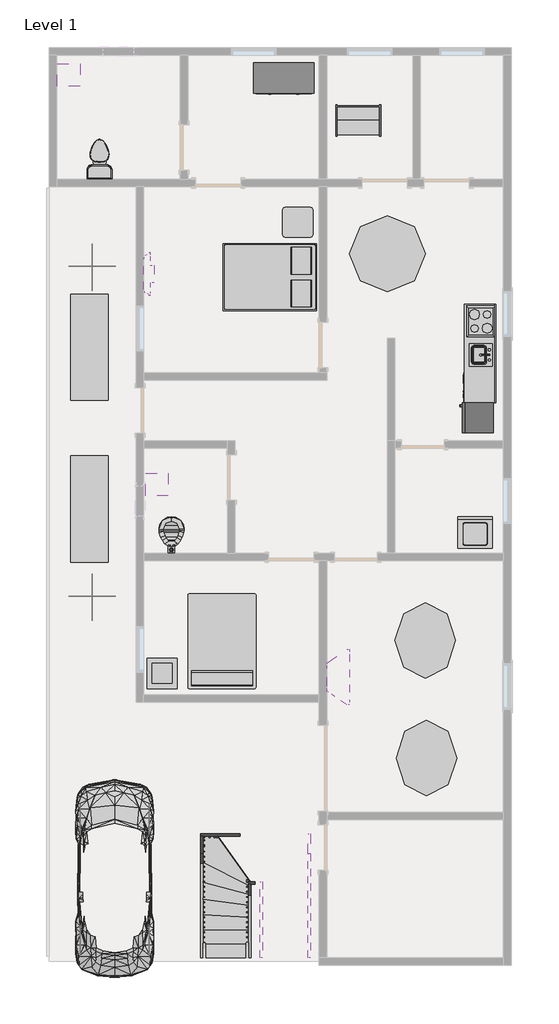
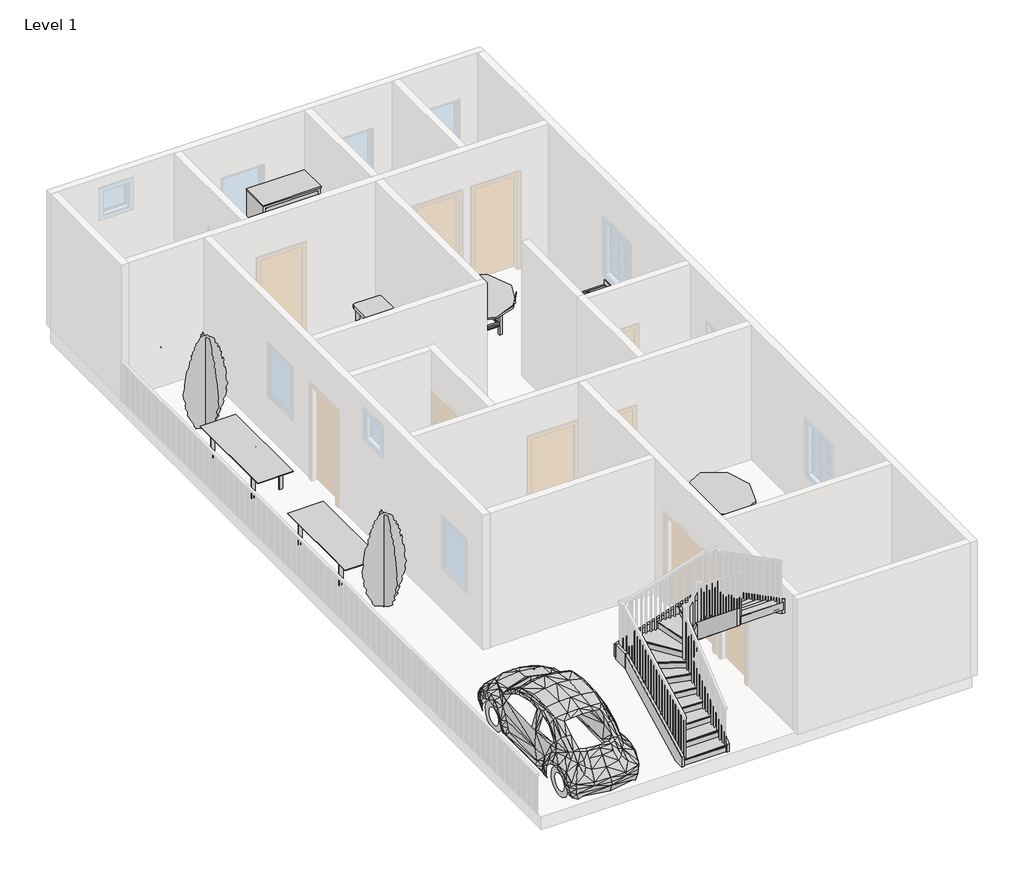
# One storey, part 4 of 4: 13 furniture elements, 8 members, 7 proxies, 5 flow terminals, 2 geographic elements, 1 stair flight.
"""IFC4 building model written with IfcOpenShell, lengths in millimetres."""

from ifc_helpers import new_model, si_unit, frame, origin, place, context, project, spatial, polyline, outline, extrude, transform, mapped, element, save
from components import proxy_a6faaae8, proxy_45b28599, kitchenette_medium_kitchenette_medium_844211aa, rpc_beetle_rpc_beetle_3ce7ba48, proxy_c523a7b7, single_carrel_single_carrel_ed4d160c, proxy_718fa39f, flow_terminal_871c2e40, flow_terminal_6d55091a, toilet_domestic_3d_toilet_domestic_3d_f7549cf7, toilet_domestic_3d_toilet_domestic_3d_183bbd19, furniture_c8abb964, furniture_0253826f, furniture_c6510c7c, furniture_9fa109b2, furniture_0810mm_56245f3a, tv_stand_tv_stand_6ce107e5, furniture_b5c51a22, furniture_92191dda, furniture_bbcc68ce, furniture_743965d2, furniture_bcf351fa, rpc_tree_conifer_0001_chinese_juniper_7_1b9786cd, stair_flight_079dc026

model = new_model("IFC4")

# Units and contexts
model_context = context("Model", 3, world=origin())
ifc_project = project(units=[si_unit("LENGTHUNIT", "METRE", prefix="MILLI")], contexts=[model_context])

# Site, building, storey
site = spatial("IfcSite", under=ifc_project)
building = spatial("IfcBuilding", under=site)
storey = spatial("IfcBuildingStorey", under=building, Name="Level 1", Elevation=0.0)

# Proxies
placement = place(None, origin())
proxy_shape = proxy_a6faaae8(model_context)
element("IfcBuildingElementProxy", 1, Name="Cook Top-4 Unit2 : 22\" x 20\"", ObjectType="Cook Top-4 Unit2 : 22\" x 20\"", at=placement, inside=storey, context=model_context, shape_type="MappedRepresentation", body=[
    mapped(proxy_shape, transform((-3348.260887, 8181.0910469, 0.0), x_axis=(0.0, -1.0, 0.0), y_axis=(1.0, 0.0, 0.0), z_axis=(0.0, 0.0, 1.0))),
])
proxy_2_shape = proxy_45b28599(model_context)
element("IfcBuildingElementProxy", 2, Name="Dishwasher : 24\" x 24\" x 34\"", ObjectType="Dishwasher : 24\" x 24\" x 34\"", at=placement, inside=storey, context=model_context, shape_type="MappedRepresentation", body=[
    mapped(proxy_2_shape, transform((-3640.1104518, 7229.9085154, 0.0), x_axis=(0.0, -1.0, 0.0), y_axis=(1.0, 0.0, 0.0), z_axis=(0.0, 0.0, 1.0))),
])
kitchenette_medium_kitchenette_medium_shape = kitchenette_medium_kitchenette_medium_844211aa(model_context)
element("IfcBuildingElementProxy", 3, Name="Kitchenette - Medium : Kitchenette - Medium", ObjectType="Kitchenette - Medium : Kitchenette - Medium", at=placement, inside=storey, context=model_context, shape_type="MappedRepresentation", body=[
    mapped(kitchenette_medium_kitchenette_medium_shape, transform((-3043.460887, 7856.9287518, 0.0), x_axis=(0.0, -1.0, 0.0), y_axis=(1.0, 0.0, 0.0), z_axis=(0.0, 0.0, 1.0))),
])
rpc_beetle_rpc_beetle_shape = rpc_beetle_rpc_beetle_3ce7ba48(model_context)
element("IfcBuildingElementProxy", 4, Name="RPC Beetle : RPC Beetle", ObjectType="RPC Beetle : RPC Beetle", at=placement, inside=storey, context=model_context, shape_type="MappedRepresentation", body=[
    mapped(rpc_beetle_rpc_beetle_shape, transform((-10714.260887, -4252.2089531, 0.0), x_axis=(1.0, 0.0, 0.0), y_axis=(0.0, 1.0, 0.0), z_axis=(0.0, 0.0, 1.0))),
])
proxy_3_shape = proxy_c523a7b7(model_context)
element("IfcBuildingElementProxy", 5, Name="Refrigerator : 24\" x 25\" LH", ObjectType="Refrigerator : 24\" x 25\" LH", at=placement, inside=storey, context=model_context, shape_type="MappedRepresentation", body=[
    mapped(proxy_3_shape, transform((-3393.9098585, 6244.3410469, 0.0), x_axis=(0.0, -1.0, 0.0), y_axis=(1.0, 0.0, 0.0), z_axis=(0.0, 0.0, 1.0))),
])
single_carrel_single_carrel_shape = single_carrel_single_carrel_ed4d160c(model_context)
element("IfcBuildingElementProxy", 6, Name="Single Carrel : Single Carrel", ObjectType="Single Carrel : Single Carrel", at=placement, inside=storey, context=model_context, shape_type="MappedRepresentation", body=[
    mapped(single_carrel_single_carrel_shape, transform((-5812.060887, 12511.7910469, 0.0), x_axis=(1.0, 0.0, 0.0), y_axis=(0.0, 1.0, 0.0), z_axis=(0.0, 0.0, 1.0))),
])
proxy_4_shape = proxy_718fa39f(model_context)
element("IfcBuildingElementProxy", 7, Name="Washer : 27\" x 25\" x 35\"", ObjectType="Washer : 27\" x 25\" x 35\"", at=placement, inside=storey, context=model_context, shape_type="MappedRepresentation", body=[
    mapped(proxy_4_shape, transform((-3882.9783555, 3660.1414821, 0.0), x_axis=(1.0, 0.0, 0.0), y_axis=(0.0, 1.0, 0.0), z_axis=(0.0, 0.0, 1.0))),
])

# Flow terminals
flow_terminal_shape = flow_terminal_871c2e40(model_context)
element("IfcFlowTerminal", 8, ObjectType="Sink Kitchen-Island : 18\" x 18\"", at=placement, inside=storey, context=model_context, shape_type="MappedRepresentation", body=[
    mapped(flow_terminal_shape, transform((-11639.0154859, 13118.4018063, 914.4), x_axis=(0.0, 1.0000000000000009, 0.0), y_axis=(-1.0000000000000009, 0.0, 0.0), z_axis=(0.0, 0.0, 1.0))),
])
element("IfcFlowTerminal", 9, ObjectType="Sink Kitchen-Island : 18\" x 18\"", at=placement, inside=storey, context=model_context, shape_type="MappedRepresentation", body=[
    mapped(flow_terminal_shape, transform((-9861.0154859, 4888.8018063, 914.4), x_axis=(0.0, 1.0000000000000009, 0.0), y_axis=(-1.0000000000000009, 0.0, 0.0), z_axis=(0.0, 0.0, 1.0))),
])
element("IfcFlowTerminal", 10, ObjectType="Sink Kitchen-Island : 18\" x 18\"", at=placement, inside=storey, context=model_context, shape_type="MappedRepresentation", body=[
    mapped(flow_terminal_shape, transform((-3350.6062881, 7523.6802875, -14.4), x_axis=(0.0, -1.0, 0.0), y_axis=(1.0, 0.0, 0.0), z_axis=(0.0, 0.0, 1.0))),
])
flow_terminal_2_shape = flow_terminal_6d55091a(model_context)
element("IfcFlowTerminal", 11, ObjectType="Toilet-Commercial-Wall-3D : 15\" Seat Height", at=placement, inside=storey, context=model_context, shape_type="MappedRepresentation", body=[
    mapped(flow_terminal_2_shape, transform((-9976.1640408, 3443.9910469, 0.0), x_axis=(1.0, 0.0, 0.0), y_axis=(0.0, 1.0, 0.0), z_axis=(0.0, 0.0, 1.0))),
])
toilet_domestic_3d_toilet_domestic_3d_shape = toilet_domestic_3d_toilet_domestic_3d_f7549cf7(model_context)
toilet_domestic_3d_toilet_domestic_3d_2_shape = toilet_domestic_3d_toilet_domestic_3d_183bbd19(model_context)
element("IfcFlowTerminal", 12, ObjectType="Toilet-Domestic-3D : Toilet-Domestic-3D", at=placement, inside=storey, context=model_context, shape_type="MappedRepresentation", body=[
    mapped(toilet_domestic_3d_toilet_domestic_3d_shape, transform((-11019.060887, 11533.2870743, 0.0), x_axis=(-1.0000000000000004, 0.0, 0.0), y_axis=(0.0, -1.0000000000000004, 0.0), z_axis=(0.0, 0.0, 1.0))),
    mapped(toilet_domestic_3d_toilet_domestic_3d_2_shape, transform((-11019.060887, 11533.2870743, 0.0), x_axis=(-1.0000000000000004, 0.0, 0.0), y_axis=(0.0, -1.0000000000000004, 0.0), z_axis=(0.0, 0.0, 1.0))),
])

# Furniture
furniture_shape = furniture_c8abb964(model_context)
element("IfcFurniture", 13, ObjectType="Bed-Box : Double 53\" x 74\"", at=placement, inside=storey, context=model_context, shape_type="MappedRepresentation", body=[
    mapped(furniture_shape, transform((-7355.6313788, 9409.2435059, 0.0), x_axis=(0.0, -1.0, 0.0), y_axis=(1.0, 0.0, 0.0), z_axis=(0.0, 0.0, 1.0))),
])
furniture_2_shape = furniture_0253826f(model_context)
element("IfcFurniture", 14, ObjectType="Bed-Standard : Double 54\" x 75\"", at=placement, inside=storey, context=model_context, shape_type="MappedRepresentation", body=[
    mapped(furniture_2_shape, transform((-8283.7723624, 1709.2959649, 0.0), x_axis=(-1.0, 0.0, 0.0), y_axis=(0.0, -1.0, 0.0), z_axis=(0.0, 0.0, 1.0))),
])
furniture_3_shape = furniture_c6510c7c(model_context)
element("IfcFurniture", 15, ObjectType="Counter Top w Sink Hole : 24\" Depth", at=placement, inside=storey, context=model_context, shape_type="MappedRepresentation", body=[
    mapped(furniture_3_shape, transform((-3043.460887, 7323.5287518, -14.4), x_axis=(0.0, -1.0, 0.0), y_axis=(1.0, 0.0, 0.0), z_axis=(0.0, 0.0, 1.0))),
])
furniture_4_shape = furniture_9fa109b2(model_context)
element("IfcFurniture", 16, ObjectType="Dresser : 48\" x 72\" x 24\"", at=placement, inside=storey, context=model_context, shape_type="MappedRepresentation", body=[
    mapped(furniture_4_shape, transform((-7041.4676272, 13433.754001, 0.0), x_axis=(1.0, 0.0, 0.0), y_axis=(0.0, 1.0, 0.0), z_axis=(0.0, 0.0, 1.0))),
])
furniture_0810mm_shape = furniture_0810mm_56245f3a(model_context)
element("IfcFurniture", 17, ObjectType="TV - Flat Screen : 32\"", at=placement, inside=storey, context=model_context, shape_type="MappedRepresentation", body=[
    mapped(furniture_0810mm_shape, transform((-10071.5222634, 9137.535561, 1219.2), x_axis=(0.0, 1.0, 0.0), y_axis=(-1.0, 0.0, 0.0), z_axis=(0.0, 0.0, 1.0))),
])
tv_stand_tv_stand_shape = tv_stand_tv_stand_6ce107e5(model_context)
element("IfcFurniture", 18, ObjectType="TV Stand : TV Stand", at=placement, inside=storey, context=model_context, shape_type="MappedRepresentation", body=[
    mapped(tv_stand_tv_stand_shape, transform((-6447.060887, 905.8030448, 1219.2), x_axis=(0.0, 1.0000000000000002, 0.0), y_axis=(-1.0000000000000002, 0.0, 0.0), z_axis=(0.0, 0.0, 1.0))),
])
furniture_5_shape = furniture_b5c51a22(model_context)
element("IfcFurniture", 19, ObjectType="Table-Coffee : 24\" x 24\" x 24\"", at=placement, inside=storey, context=model_context, shape_type="MappedRepresentation", body=[
    mapped(furniture_5_shape, transform((-9780.0266537, 1011.9799691, 0.0), x_axis=(1.0, 0.0, 0.0), y_axis=(0.0, 1.0, 0.0), z_axis=(0.0, 0.0, 1.0))),
])
furniture_6_shape = furniture_92191dda(model_context)
element("IfcFurniture", 20, ObjectType="Table-Dining : 30\" x 84\" x 22\"", at=placement, inside=storey, context=model_context, shape_type="MappedRepresentation", body=[
    mapped(furniture_6_shape, transform((-11127.0498092, 4390.9252802, 0.0), x_axis=(0.0, 1.0000000000000002, 0.0), y_axis=(-1.0000000000000002, 0.0, 0.0), z_axis=(0.0, 0.0, 1.0))),
])
element("IfcFurniture", 21, ObjectType="Table-Dining : 30\" x 84\" x 22\"", at=placement, inside=storey, context=model_context, shape_type="MappedRepresentation", body=[
    mapped(furniture_6_shape, transform((-11127.0498092, 7642.1252802, 0.0), x_axis=(0.0, 1.0000000000000002, 0.0), y_axis=(-1.0000000000000002, 0.0, 0.0), z_axis=(0.0, 0.0, 1.0))),
])
furniture_7_shape = furniture_bbcc68ce(model_context)
element("IfcFurniture", 22, ObjectType="Table-Dining Round w Chairs : 60\" Diameter", at=placement, inside=storey, context=model_context, shape_type="MappedRepresentation", body=[
    mapped(furniture_7_shape, transform((-5331.5428542, 9724.8697354, 0.0), x_axis=(1.0, 0.0, 0.0), y_axis=(0.0, 1.0, 0.0), z_axis=(0.0, 0.0, 1.0))),
])
furniture_8_shape = furniture_743965d2(model_context)
element("IfcFurniture", 23, ObjectType="Table-Ellipse : 60\" x 48\"", at=placement, inside=storey, context=model_context, shape_type="MappedRepresentation", body=[
    mapped(furniture_8_shape, transform((-4465.860887, 1767.5910469, 0.0), x_axis=(0.0, 1.0000000000000002, 0.0), y_axis=(-1.0000000000000002, 0.0, 0.0), z_axis=(0.0, 0.0, 1.0))),
])
element("IfcFurniture", 24, ObjectType="Table-Ellipse : 60\" x 48\"", at=placement, inside=storey, context=model_context, shape_type="MappedRepresentation", body=[
    mapped(furniture_8_shape, transform((-4440.460887, -594.6089531, 0.0), x_axis=(0.0, 1.0000000000000002, 0.0), y_axis=(-1.0000000000000002, 0.0, 0.0), z_axis=(0.0, 0.0, 1.0))),
])
furniture_9_shape = furniture_bcf351fa(model_context)
element("IfcFurniture", 25, ObjectType="Table-End : 24\" x 24\"", at=placement, inside=storey, context=model_context, shape_type="MappedRepresentation", body=[
    mapped(furniture_9_shape, transform((-7339.7945173, 10022.5910469, 0.0), x_axis=(1.0, 0.0, 0.0), y_axis=(0.0, 1.0, 0.0), z_axis=(0.0, 0.0, 1.0))),
])

# Geographic elements
rpc_tree_conifer_0001_chinese_juniper_7_shape = rpc_tree_conifer_0001_chinese_juniper_7_1b9786cd(model_context)
element("IfcGeographicElement", 26, ObjectType="RPC Tree - Conifer.0001 : Chinese Juniper - 7'", at=placement, inside=storey, context=model_context, shape_type="MappedRepresentation", body=[
    mapped(rpc_tree_conifer_0001_chinese_juniper_7_shape, transform((-11171.6575581, 9285.9910469, 0.0), x_axis=(1.0, 0.0, 0.0), y_axis=(0.0, 1.0, 0.0), z_axis=(0.0, 0.0, 1.0))),
])
element("IfcGeographicElement", 27, ObjectType="RPC Tree - Conifer.0001 : Chinese Juniper - 7'", at=placement, inside=storey, context=model_context, shape_type="MappedRepresentation", body=[
    mapped(rpc_tree_conifer_0001_chinese_juniper_7_shape, transform((-11171.6575581, 2656.5910469, 0.0), x_axis=(1.0, 0.0, 0.0), y_axis=(0.0, 1.0, 0.0), z_axis=(0.0, 0.0, 1.0))),
])

# Members
element("IfcMember", 28, ObjectType="Stringer - 2\" Width", at=placement, inside=storey, context=model_context, shape_type="SweptSolid", body=[
    extrude(outline(polyline([(-4607.8089531, 0.0), (-4607.8089531, 229.639954), (-2520.3917614, 1305.3956453), (-2520.3917614, 962.500629), (-4388.0466355, 0.0), (-4607.8089531, 0.0)])), frame((-8987.060887, 0.0, 0.0), z_axis=(1.0, 0.0, 0.0), x_axis=(0.0, 1.0, 0.0)), (0.0, 0.0, 1.0), 50.8),
])
element("IfcMember", 29, ObjectType="Stringer - 2\" Width", at=placement, inside=storey, context=model_context, shape_type="SweptSolid", body=[
    extrude(outline(polyline([(-8936.260887, -2520.3917614), (-8987.060887, -2520.3917614), (-8987.060887, -2165.6772612), (-8936.260887, -2165.6772612), (-8936.260887, -2520.3917614)])), frame((0.0, 0.0, 962.500629), z_axis=(0.0, 0.0, 1.0), x_axis=(1.0, 0.0, 0.0)), (0.0, 0.0, 1.0), 342.8950162),
])
element("IfcMember", 30, ObjectType="Stringer - 2\" Width", at=placement, inside=storey, context=model_context, shape_type="SweptSolid", body=[
    extrude(outline(polyline([(1289.0952212, -8987.060887), (1000.5956453, -8987.060887), (1000.5956453, -8817.5384041), (1638.9682298, -6828.060887), (1969.9972697, -6828.060887), (1969.9972697, -6865.0410043), (1289.0952212, -8987.060887)])), frame((0.0, -2165.6772612, 0.0), z_axis=(0.0, 1.0, 0.0), x_axis=(0.0, 0.0, 1.0)), (0.0, 0.0, 1.0), 50.8),
])
element("IfcMember", 31, ObjectType="Stringer - 2\" Width", at=placement, inside=storey, context=model_context, shape_type="SweptSolid", body=[
    extrude(outline(polyline([(-6828.060887, -2114.8772612), (-6777.260887, -2114.8772612), (-6777.260887, -2520.3917614), (-6828.060887, -2520.3917614), (-6828.060887, -2114.8772612)])), frame((0.0, 0.0, 1649.8904473), z_axis=(0.0, 0.0, 1.0), x_axis=(1.0, 0.0, 0.0)), (0.0, 0.0, 1.0), 320.1068224),
])
element("IfcMember", 32, ObjectType="Stringer - 2\" Width", at=placement, inside=storey, context=model_context, shape_type="SweptSolid", body=[
    extrude(outline(polyline([(-2520.3917614, 1969.9972697), (-2520.3917614, 1649.8904473), (-4607.8089531, 2725.6461385), (-4607.8089531, 3045.7529609), (-2520.3917614, 1969.9972697)])), frame((-6828.060887, 0.0, 0.0), z_axis=(1.0, 0.0, 0.0), x_axis=(0.0, 1.0, 0.0)), (0.0, 0.0, 1.0), 50.8),
])
element("IfcMember", 33, ObjectType="Stringer - 2\" Width", at=placement, inside=storey, context=model_context, shape_type="SweptSolid", body=[
    extrude(outline(polyline([(-4607.8089531, 0.0), (-4607.8089531, 176.1764461), (-3130.8772612, 1380.418648), (-3130.8772612, 987.1410923), (-4341.5473085, 0.0), (-4607.8089531, 0.0)])), frame((-8021.860887, 0.0, 0.0), z_axis=(1.0, 0.0, 0.0), x_axis=(0.0, 1.0, 0.0)), (0.0, 0.0, 1.0), 50.8),
])
element("IfcMember", 34, ObjectType="Stringer - 2\" Width", at=placement, inside=storey, context=model_context, shape_type="SweptSolid", body=[
    extrude(outline(polyline([(1573.2682978, -8021.860887), (1028.5617647, -8021.860887), (1028.5617647, -7987.6186697), (1360.465107, -7793.260887), (1926.1409689, -7793.260887), (1926.1409689, -7815.2237696), (1573.2682978, -8021.860887)])), frame((0.0, -3130.8772612, 0.0), z_axis=(0.0, 1.0, 0.0), x_axis=(0.0, 0.0, 1.0)), (0.0, 0.0, 1.0), 50.8),
])
element("IfcMember", 35, ObjectType="Stringer - 2\" Width", at=placement, inside=storey, context=model_context, shape_type="SweptSolid", body=[
    extrude(outline(polyline([(-3080.0772612, 1926.1409689), (-3080.0772612, 1532.8634131), (-4607.8089531, 2778.5262875), (-4607.8089531, 3171.8038432), (-3080.0772612, 1926.1409689)])), frame((-7793.260887, 0.0, 0.0), z_axis=(1.0, 0.0, 0.0), x_axis=(0.0, 1.0, 0.0)), (0.0, 0.0, 1.0), 50.8),
])

# Stair flight
stair_flight_shape = stair_flight_079dc026(model_context)
element("IfcStairFlight", 36, ObjectType="2\" Tread 1\" Nosing 1/4\" Riser", at=placement, inside=storey, context=model_context, shape_type="MappedRepresentation", body=[
    mapped(stair_flight_shape, transform((0.0, 0.0, 0.0), x_axis=(1.0, 0.0, 0.0), y_axis=(0.0, 1.0, 0.0), z_axis=(0.0, 0.0, 1.0))),
])

save(model, "model.ifc")

# Revit data of these elements
# Type "Cook Top-4 Unit2 : 22\" x 20\""
#   Depth = 1' - 8"
#   Width = 1' - 10"
#   Burner Material = Steel, Chrome Plated
#   Cooktop Material = Steel, Polished
#   Default Elevation = 0
#   Assembly Code = ""
# Type "Dishwasher : 24\" x 24\" x 34\""
#   Label = "DW"
#   Assembly Code = "E1090400"
#   Depth = 2' - 0"
#   Height = 2' - 10"
#   Width = 2' - 0"
#   Dishwasher Material = Steel, Paint Finish, Ivory, Glossy
#   Panel Face Material = Plastic, Opaque Black
#   Default Elevation = 0
# Type "Kitchenette - Medium : Kitchenette - Medium"
#   Assembly Code = "E1090400"
#   Counter Length = 6' - 6"
#   Cabinet Width = 4' - 6"
#   Cabinet Height = 2' - 10 1/2"
#   Cabinet Depth = 2' - 0"
#   Toe Depth = 0' - 3"
#   Toe Height = 0' - 3 1/2"
#   Cabinet Material = Cabinets
#   Door/Drawer Material = Cabinets
#   Handle Material = Cabinets - Handles
#   Default Elevation = 0
# Type "RPC Beetle : RPC Beetle"
#   built-in parameter 1005195 = "RPC-16-0U6E-L4EG-ENH1-J3KF-SVEL-0TX4-C0"
#   Height = 0
# Type "Refrigerator : 24\" x 25\" LH"
#   Label = "REF."
#   Assembly Code = "E1090400"
#   Depth = 2' - 0 3/4"
#   Handle = 0' - 1 1/2"
#   Height = 5' - 3 1/2"
#   Rear Clearance = 0' - 2"
#   Top Door Height = 1' - 8"
#   Width = 1' - 11 1/2"
#   Material = Steel, Paint Finish, Ivory, Glossy
#   Default Elevation = 0
# Type "Single Carrel : Single Carrel"
#   Assembly Code = "E1020200"
#   Width = 2' - 11 3/4"
#   Carrel Material = Laminate, Ivory, Matte
#   Desktop/Shelf Material = Cherry
#   Default Elevation = 0
# Type "Washer : 27\" x 25\" x 35\""
#   Label = "W"
#   Assembly Code = "E1090400"
#   Depth = 2' - 1"
#   Height = 2' - 11"
#   Width = 2' - 3"
#   Washer Material = Steel, Paint Finish, Ivory, Matte
#   Default Elevation = 0
# Type "Sink Kitchen-Island : 18\" x 18\""
#   Assembly Code = "D2010410"
#   Counter Height = 3' - 0"
#   Depth = 1' - 6"
#   Width = 1' - 6"
#   Faucet Material = Steel, Polished
#   Sink Material = Steel, Polished
#   Default Elevation = 0
# Type "Toilet-Commercial-Wall-3D : 15\" Seat Height"
#   Assembly Code = "D2010110"
#   Mounting Height = 1' - 3"
#   Piping Material = Steel, Polished
#   Toilet - Bowl Material = Porcelain, Ivory
#   Toilet - Seat Material = Laminate, Ivory, Matte
#   Default Elevation = 0
# Type "Toilet-Domestic-3D : Toilet-Domestic-3D"
#   Assembly Code = "D2010110"
#   Toilet - Bowl/Basin Material = Porcelain, Linen
#   Toilet - Seat Material = Laminate, Linen, Matte
#   Default Elevation = 0
# Type "Bed-Box : Double 53\" x 74\""
#   Assembly Code = "E2020200"
#   Length = 6' - 2"
#   Width = 4' - 5"
#   Frame Material = Birch
#   Mattress Material = Linen, White
#   Default Elevation = 0
# Type "Bed-Standard : Double 54\" x 75\""
#   Assembly Code = "E2020200"
#   Length = 6' - 3"
#   Width = 4' - 6"
#   Leg Material = Steel, Chrome Plated
#   Mattress Material = Linen, White
#   Default Elevation = 0
# Type "Counter Top w Sink Hole : 24\" Depth"
#   Assembly Code = "C1030400"
#   Counter Thickness = 0' - 1 1/2"
#   Depth = 2' - 1"
#   Height = 3' - 0"
#   Length [instance default] = 8' - 0"
#   Sink Location [instance default] = 2' - 0"
#   Sink Location To Wall [instance default] = 0' - 6"
#   Sink Opening Depth [instance default] = 1' - 3"
#   Sink Opening Width [instance default] = 2' - 3"
#   Counter Top Material = none
#   Default Elevation = 0
# Type "Dresser : 48\" x 72\" x 24\""
#   Assembly Code = "E2020200"
#   Depth = 2' - 0"
#   Height = 6' - 0"
#   Width = 4' - 0"
#   Dresser Material = Laminate - Ivory, Glossy
#   Drawer Material = Laminate, Ivory, Matte
#   Knob Material = Cherry
#   Default Elevation = 0
# Type "TV - Flat Screen : 32\""
#   SinAng = 0' - 0.0193"
#   L = 2' - 3.79372"
#   H = 1' - 3.6354"
#   Thickness = 0' - 4.33071"
#   Diagonal = 2' - 7.88976"
#   CosAng = 0' - 0.03431"
#   Stand [instance default] = yes
#   Default Elevation = 0
# Type "TV Stand : TV Stand"
#   Depth = 1' - 6"
#   Width = 3' - 8"
#   Height = 1' - 7 1/2"
#   Finish = Melamine - Gray
#   Default Elevation = 0
# Type "Table-Coffee : 24\" x 24\" x 24\""
#   Assembly Code = "E2020200"
#   Height = 2' - 0"
#   Length = 2' - 0"
#   Width = 2' - 0"
#   Top Material = none
#   Frame Material = none
#   Default Elevation = 0
# Type "Table-Dining : 30\" x 84\" x 22\""
#   Assembly Code = "E2020200"
#   Height = 1' - 10"
#   Length = 7' - 0"
#   Width = 2' - 6"
#   Base Material = Steel, Chrome Plated
#   Top Material = Glass - Clear, Grey
#   Default Elevation = 0
# Type "Table-Dining Round w Chairs : 60\" Diameter"
#   Assembly Code = "E2020200"
#   Radius = 2' - 6"
#   Diameter = 5' - 0"
#   Height = 2' - 6"
#   Chairs = 6
#   Base Material = Pine
#   Top Material = Laminate, Linen, Matte
#   Default Elevation = 0
# Type "Table-Ellipse : 60\" x 48\""
#   Assembly Code = "E2020200"
#   Half Width = 2' - 0"
#   Half Length = 2' - 6"
#   Height = 2' - 6"
#   Length = 5' - 0"
#   Width = 4' - 0"
#   Base Material = Birch
#   Top Material = Birch
#   Default Elevation = 0
# Type "Table-End : 24\" x 24\""
#   Assembly Code = "E2020200"
#   Height = 2' - 6"
#   Length = 2' - 0"
#   Width = 2' - 0"
#   Base Material = Birch
#   Top Material = Laminate, Ivory, Matte
#   Default Elevation = 0
# Type "RPC Tree - Conifer.0001 : Chinese Juniper - 7'"
#   built-in parameter 1005198 = "{2, 15},{39, RPC-16-FUM3-UUQ0-UBF0-N000-ST1L-LVER-AU},{1, 0},{1, 0},{2, 13},{1, 8},{5, Color},{1, 0},{1, 0},{3, 0.8},{3, 0.8},{3, 0.8},{1, 8},{7, BBoxMin},{1, 0},{1, 0},{1, 0},{1, 0},{1, 0},{1, 8},{7, BBoxMax},{1, 0},{1, 0},{1, 0},{1, 0},{1, 0},{2, 11},{9, RPCTypeId},{1, 0},{1, 0},{39, RPC-16-FUM3-UUQ0-UBF0-N000-ST1L-LVER-AU},{1, 6},{14, RPCPlantHeight},{1, 0},{1, 0},{1, 7},{2, 11},{7, keyword},{1, 0},{1, 0},{34, :RPCs:Trees [General]:Geometry:RPC},{2, 11},{8, category},{1, 0},{1, 0},{15, Trees [General]},{2, 11},{12, LocalizedUID},{1, 0},{1, 0},{15, Chinese Juniper},{2, 14},{6, Height},{1, 0},{1, 0},{1, 7},{1, 2},{16, Cast Reflections},{1, 0},{1, 0},{1, 0},{1, 2},{12, Cast Shadows},{1, 0},{1, 0},{1, 1},{1, 2},{9, Lock View},{1, 0},{1, 0},{1, 0},{1, 4},{5, ViewC},{1, 0},{1, 0},{1, 0},{21, assetlibrary_base.fbx},{1, 5},"
#   built-in parameter 1005195 = "RPC-16-FUM3-UUQ0-UBF0-N000-ST1L-LVER-AU"
#   Type Comments = "Chinese Juniper"
#   Assembly Code = "G2050500"
#   Height = 7' - 0"
#   Description = (empty or 0)
#   Default Elevation = 0
# Element 1 (IfcBuildingElementProxy, "Cook Top-4 Unit2 : 22\" x 20\"")
#   Phase Created = New Construction
#   Materials on its faces: "Steel, Chrome Plated", "Steel, Polished"
# Element 2 (IfcBuildingElementProxy, "Dishwasher : 24\" x 24\" x 34\"")
#   Phase Created = New Construction
#   Materials on its faces: "Steel, Paint Finish, Ivory, Glossy", "Plastic, Opaque Black"
# Element 3 (IfcBuildingElementProxy, "Kitchenette - Medium : Kitchenette - Medium")
#   Phase Created = New Construction
#   Materials on its faces: "Cabinets", "Cabinets - Handles"
# Element 4 (IfcBuildingElementProxy, "RPC Beetle : RPC Beetle")
#   Phase Created = New Construction
# Element 5 (IfcBuildingElementProxy, "Refrigerator : 24\" x 25\" LH")
#   Phase Created = New Construction
#   Materials on its faces: "Steel, Paint Finish, Ivory, Glossy", "Steel, Chrome Plated"
# Element 6 (IfcBuildingElementProxy, "Single Carrel : Single Carrel")
#   Phase Created = New Construction
#   Materials on its faces: "Laminate, Ivory, Matte", "Cherry"
# Element 7 (IfcBuildingElementProxy, "Washer : 27\" x 25\" x 35\"")
#   Phase Created = New Construction
#   Materials on its faces: "Steel, Paint Finish, Ivory, Matte"
# Element 8 (IfcFlowTerminal, "Sink Kitchen-Island : 18\" x 18\"")
#   Mark = "2"
#   Phase Created = New Construction
#   Materials on its faces: "Steel, Polished"
# Element 9 (IfcFlowTerminal, "Sink Kitchen-Island : 18\" x 18\"")
#   Mark = "5"
#   Phase Created = New Construction
#   Materials on its faces: "Steel, Polished"
# Element 10 (IfcFlowTerminal, "Sink Kitchen-Island : 18\" x 18\"")
#   Mark = "15"
#   Phase Created = New Construction
#   Materials on its faces: "Steel, Polished"
# Element 11 (IfcFlowTerminal, "Toilet-Commercial-Wall-3D : 15\" Seat Height")
#   Mark = "4"
#   Phase Created = New Construction
#   Materials on its faces: "Laminate, Ivory, Matte", "Porcelain, Ivory", "Steel, Polished"
# Element 12 (IfcFlowTerminal, "Toilet-Domestic-3D : Toilet-Domestic-3D")
#   Mark = "1"
#   Phase Created = New Construction
#   Materials on its faces: "Porcelain, Linen", "Laminate, Linen, Matte"
# Element 13 (IfcFurniture, "Bed-Box : Double 53\" x 74\"")
#   Phase Created = New Construction
#   Materials on its faces: "Birch", "Linen, White"
# Element 14 (IfcFurniture, "Bed-Standard : Double 54\" x 75\"")
#   Phase Created = New Construction
#   Materials on its faces: "Linen, White", "Steel, Chrome Plated"
# Element 15 (IfcFurniture, "Counter Top w Sink Hole : 24\" Depth")
#   Sink Opening Depth = 1' - 2"
#   Sink Location To Wall = 0' - 6"
#   Length = 6' - 6"
#   Sink Location = 3' - 4"
#   Sink Opening Width = 1' - 4"
#   Phase Created = New Construction
#   Materials on its faces: "Counter Top"
# Element 16 (IfcFurniture, "Dresser : 48\" x 72\" x 24\"")
#   Phase Created = New Construction
#   Materials on its faces: "Laminate, Ivory, Matte", "Cherry", "Laminate - Ivory, Glossy"
# Element 17 (IfcFurniture, "TV - Flat Screen : 32\"")
#   Stand = yes
#   Phase Created = New Construction
#   Materials on its faces: "TV - Black", "TV - Glass", "TV - Screen"
# Element 18 (IfcFurniture, "TV Stand : TV Stand")
#   Phase Created = New Construction
#   Materials on its faces: "Melamine - Gray", "Glass - Shelves"
# Element 19 (IfcFurniture, "Table-Coffee : 24\" x 24\" x 24\"")
#   Phase Created = New Construction
#   Materials on its faces: "Glass - Clear, Grey"
# Elements 20, 21 (IfcFurniture, "Table-Dining : 30\" x 84\" x 22\"")
#   Phase Created = New Construction
#   Materials on its faces: "Steel, Chrome Plated", "Glass - Clear, Grey"
# Element 22 (IfcFurniture, "Table-Dining Round w Chairs : 60\" Diameter")
#   Phase Created = New Construction
#   Materials on its faces: "Pine", "Laminate, Linen, Matte"
# Elements 23, 24 (IfcFurniture, "Table-Ellipse : 60\" x 48\"")
#   Phase Created = New Construction
#   Materials on its faces: "Birch"
# Element 25 (IfcFurniture, "Table-End : 24\" x 24\"")
#   Phase Created = New Construction
#   Materials on its faces: "Laminate, Ivory, Matte", "Birch"
# Elements 26, 27 (IfcGeographicElement, "RPC Tree - Conifer.0001 : Chinese Juniper - 7'")
#   Phase Created = New Construction
# Elements 28, 29, 30, 31, 32, 33, 34, 35 (IfcMember, "Stringer - 2\" Width")
#   Phase Created = New Construction
# Element 36 (IfcStairFlight, "2\" Tread 1\" Nosing 1/4\" Riser")
#   Phase Created = New Construction
# Materials
#   "Steel, Chrome Plated": class "Metal", colour RGB 17 17 17, transparency 0, Description = "Chromiuim plated steel", Cost = 0
#   "Steel, Polished": class "Metal", colour RGB 57 57 57, transparency 0, Description = "Polished steel", Cost = 0
#   "Steel, Paint Finish, Ivory, Glossy": class "Metal", colour RGB 247 247 239, transparency 0, Description = "Steel, paint finish, ivory, glossy", Cost = 0
#   "Plastic, Opaque Black": class "Plastic", colour RGB 0 0 0, transparency 0.7, Description = "Plastic, generic, opaque black", Cost = 0
#   "Cabinets": colour RGB 249 249 249, transparency 0
#   "Cabinets - Handles": class "Metal", colour RGB 57 57 57, transparency 0
#   "Laminate, Ivory, Matte": class "Plastic", colour RGB 247 247 239, transparency 0, Description = "Plastic Laminate - Ivory, Matte", Cost = 0
#   "Cherry": class "Wood", colour RGB 226 177 128, transparency 0, Description = "Prunus Serotina", Cost = 0
#   "Steel, Paint Finish, Ivory, Matte": class "Metal", colour RGB 247 247 239, transparency 0, Description = "Steel, paint finish, ivory, matte", Cost = 0
#   "Porcelain, Ivory": class "Ceramic", colour RGB 247 247 239, transparency 0, Description = "Porcelain, ivory", Cost = 0
#   "Porcelain, Linen": class "Ceramic", colour RGB 249 239 230, transparency 0, Description = "Porcelain, linen", Cost = 0
#   "Laminate, Linen, Matte": class "Plastic", colour RGB 249 239 230, transparency 0, Description = "Plastic Laminate - Linen, Matte", Cost = 0
#   "Birch": class "Wood", colour RGB 224 178 126, transparency 0, Description = "Betula Alleghaniensis", Cost = 0
#   "Linen, White": class "Textile", colour RGB 247 247 239, transparency 0, Description = "Linen, white", Cost = 0
#   "Laminate - Ivory, Glossy": colour RGB 247 247 239, transparency 0
#   "Melamine - Gray": class "Wood", colour RGB 49 49 49, transparency 0
#   "Glass - Clear, Grey": class "Glass", colour RGB 252 255 255, transparency 0.64
#   "Pine": class "Wood", colour RGB 223 192 134, transparency 0, Description = "Pinus Echinata", Cost = 0
#   "Counter Top": class "Wood", colour RGB 226 177 128, transparency 0
#   "TV - Black": colour RGB 49 49 49, transparency 0
#   "TV - Glass": colour RGB 157 157 157, transparency 0.9
#   "TV - Screen": colour RGB 0 0 0, transparency 0
#   "Glass - Shelves": class "Glass", colour RGB 167 167 167, transparency 0.9
